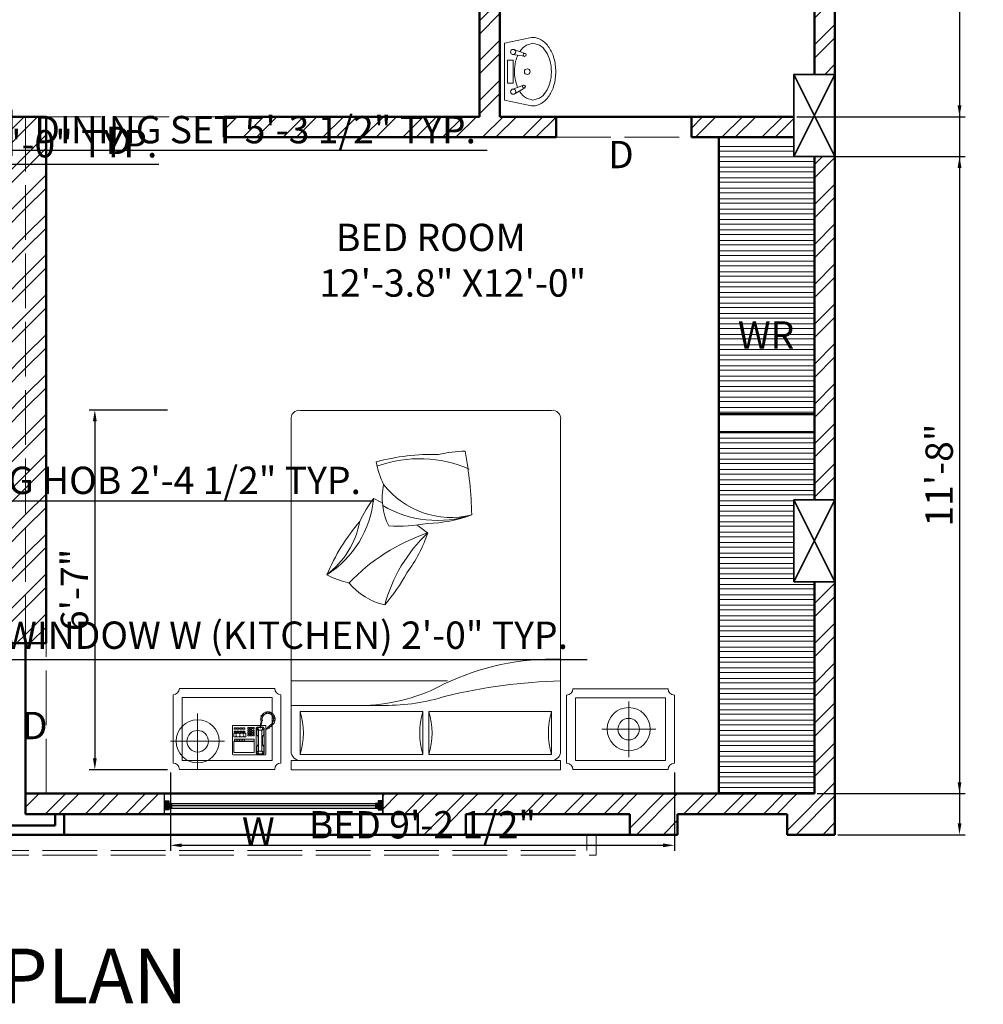
# Model space of a CAD drawing. Units: millimetres. Extents: x 4237 to 5109, y 21391 to 22486.
# Tile 14 of 17: x 4894 to 5105, y 21940 to 22156. Entities that reach past the tile are written whole.
import ezdxf

# ---------------------------------------------------------------- set-up
doc = ezdxf.new("R2010")
doc.units = ezdxf.units.MM
doc.linetypes.add('ACAD_ISO02W100', pattern=[15, 12, -3])
for name, color, linetype, lineweight in [('A-ANNO-DIMS', 2, 'Continuous', 18), ('A-ANNO-TEXT', 7, 'Continuous', 18), ('A-AREA-IDEN', 3, 'Continuous', 18), ('A-FLOR-OVHD', 1, 'ACAD_ISO02W100', 18), ('A-FURN', 8, 'Continuous', 18), ('A-FURN-CASE', 31, 'Continuous', 13), ('A-WALL', 7, 'Continuous', 50), ('A-WALL-PATT', 252, 'Continuous', 13), ('column', 102, 'Continuous', 35), ('windows', 140, 'Continuous', 25)]:
    doc.layers.add(name, color=color, linetype=linetype, lineweight=lineweight)
doc.styles.get("Standard").update_dxf_attribs({"font": 'arial.ttf'})
doc.dimstyles.new('ISO-25', dxfattribs={"dimtxt": 6, "dimasz": 2.5, "dimexe": 1.25, "dimexo": 0.625, "dimtad": 1, "dimdec": 1, "dimlunit": 4, "dimtxsty": 'Standard', "dimcen": 2.5, "dimadec": 0, "dimazin": 0, "dimtfac": 1, "dimtdec": 1, "dimtmove": 0, "dimatfit": 3, "dimfxl": 1, "dimarcsym": 0})

# ---------------------------------------------------------------- blocks, each defined once
blk = doc.blocks.new('A$C60F95712')
for p, q in [((0.05, 0.45), (0.003, 0.2283)), ((0.55, 0.45), (0.05, 0.45)), ((0.597, 0.2283), (0.55, 0.45)), ((0.1035, 0.3639), (0.1588, 0.2727)), ((0.1448, 0.3831), (0.1814, 0.2836)), ((0.4, 0.425), (0.2, 0.425)), ((0.2, 0.425), (0.2, 0.375)), ((0.2, 0.375), (0.4, 0.375)), ((0.4, 0.375), (0.4, 0.425)), ((0.4514, 0.3804), (0.4348, 0.2751)), ((0.4953, 0.3684), (0.459, 0.2688))]:
    blk.add_line(p, q)
for points in [[(0.4439, 0.3328, 0.046779), (0.3911, 0.3524, 0.080145), (0.3, 0.3617, 0.065516), (0.2003, 0.3485, 0.037125), (0.1623, 0.3353, 0.107176)], [(0.1307, 0.319, 0.008163), (0.1232, 0.3143, 0.107176), (0.0669, 0.2578), (0.05, 0.2), (0.0669, 0.1422, 0.107176), (0.1232, 0.0857, 0.078233), (0.2003, 0.0515, 0.065516), (0.3, 0.0383, 0.065516), (0.3997, 0.0515, 0.078233), (0.4768, 0.0857, 0.107176), (0.5331, 0.1422), (0.55, 0.2)], [(0.55, 0.2), (0.5331, 0.2578, 0.107176), (0.4768, 0.3143, 0.000976), (0.4758, 0.3149, 0.080145)]]:
    blk.add_lwpolyline(points, format="xyb")
for centre, radius in [((0.1241, 0.3735), 0.0228), ((0.4733, 0.3744), 0.0228), ((0.1696, 0.2793), 0.0126), ((0.3, 0.25), 0.025), ((0.4472, 0.2731), 0.0126)]:
    blk.add_circle(centre, radius)
for centre, radius, start, end in [((0.1362, 0.2), 0.1362, 168.02396, 180), ((0.1362, 0.2), 0.1362, 180, 211.85353), ((0.4638, 0.2), 0.1362, 328.14647, 0), ((0.4638, 0.2), 0.1362, 0, 11.97604), ((0.2147, 0.2488), 0.2286, 211.85353, 236.30993), ((0.3853, 0.2488), 0.2286, 303.69007, 328.14647), ((0.2662, 0.3261), 0.3215, 236.30993, 254.56292), ((0.3, 0.4484), 0.4484, 254.56292, 270), ((0.3, 0.4484), 0.4484, 270, 285.43708), ((0.3338, 0.3261), 0.3215, 285.43708, 303.69007)]:
    blk.add_arc(centre, radius, start, end)
blk = doc.blocks.new('A$C07097A50')
for p, q in [((0.0503, 1.9981), (0.5803, 1.9981)), ((0.1513, 1.6872), (0.1513, 1.9968)), ((0.6716, 1.9489), (0.6716, 2.0001)), ((0.6716, 2.0001), (2.1719, 2.0001)), ((2.1719, 1.9489), (2.1719, 2.0001)), ((2.7701, 1.9993), (2.2401, 1.9993)), ((0.0153, 1.9631), (0.0153, 1.5831)), ((0.0653, 1.9481), (0.0653, 1.5981)), ((0.0653, 1.9481), (0.5653, 1.9481)), ((0.5653, 1.9481), (0.5653, 1.5981)), ((0.6153, 1.9631), (0.6153, 1.5831)), ((2.1719, 1.9489), (0.6716, 1.9489)), ((2.2051, 1.9643), (2.2051, 1.5843)), ((2.2551, 1.9493), (2.2551, 1.5993)), ((2.7551, 1.9493), (2.2551, 1.9493)), ((2.5505, 1.6201), (2.5505, 1.9296)), ((2.7551, 1.9493), (2.7551, 1.5993)), ((2.8051, 1.9643), (2.8051, 1.5843)), ((0.3481, 1.9163), (0.3458, 1.914)), ((0.3458, 1.914), (0.3458, 1.7563)), ((0.3481, 1.9163), (0.5287, 1.9163)), ((0.3526, 1.9037), (0.3526, 1.8431)), ((0.4669, 1.9037), (0.3526, 1.9037)), ((0.4669, 1.8431), (0.4669, 1.9037)), ((0.4772, 1.9071), (0.4818, 1.9129)), ((0.4772, 1.7688), (0.4772, 1.9071)), ((0.4818, 1.9094), (0.4807, 1.9049)), ((0.4807, 1.9049), (0.4807, 1.874)), ((0.4807, 1.9049), (0.4909, 1.8946)), ((0.4807, 1.874), (0.4829, 1.8683)), ((0.4818, 1.9129), (0.5161, 1.9129)), ((0.4864, 1.9117), (0.4818, 1.9094)), ((0.4829, 1.8683), (0.4864, 1.8626)), ((0.4921, 1.8969), (0.4864, 1.9117)), ((0.4864, 1.9117), (0.5138, 1.9117)), ((0.4909, 1.8946), (0.4921, 1.8969)), ((0.4909, 1.8431), (0.4909, 1.8946)), ((0.5081, 1.8969), (0.4921, 1.8969)), ((0.5081, 1.8969), (0.5138, 1.9117)), ((0.5092, 1.8946), (0.5081, 1.8969)), ((0.5195, 1.9049), (0.5092, 1.8946)), ((0.5092, 1.8431), (0.5092, 1.8946)), ((0.5138, 1.9117), (0.5184, 1.9094)), ((0.5172, 1.8683), (0.5138, 1.8626)), ((0.5161, 1.9129), (0.5218, 1.9071)), ((0.5195, 1.874), (0.5172, 1.8683)), ((0.5184, 1.9094), (0.5195, 1.9049)), ((0.5195, 1.9049), (0.5195, 1.874)), ((0.5218, 1.9071), (0.5218, 1.77)), ((0.5287, 1.9163), (0.5309, 1.914)), ((0.5309, 1.914), (0.5309, 1.7563)), ((0.6716, 1.8977), (0.6716, 0.0512)), ((2.1719, 0.0512), (2.1719, 1.8977)), ((0, 1.8416), (0.3001, 1.8416)), ((0.3526, 1.8431), (0.4669, 1.8431)), ((0.4201, 1.8168), (0.3526, 1.8168)), ((0.3526, 1.8168), (0.3526, 1.7963)), ((0.3572, 1.8409), (0.3572, 1.8294)), ((0.4669, 1.8409), (0.3572, 1.8409)), ((0.3572, 1.8294), (0.4669, 1.8294)), ((0.3675, 1.8146), (0.3641, 1.8146)), ((0.3641, 1.8146), (0.3641, 1.8111)), ((0.3641, 1.8111), (0.3675, 1.8111)), ((0.3664, 1.8409), (0.3664, 1.8294)), ((0.3675, 1.8111), (0.3675, 1.8146)), ((0.3755, 1.8409), (0.3755, 1.8294)), ((0.3846, 1.8409), (0.3846, 1.8294)), ((0.3846, 1.8146), (0.3846, 1.8111)), ((0.3881, 1.8146), (0.3846, 1.8146)), ((0.3846, 1.8111), (0.3881, 1.8111)), ((0.3881, 1.8111), (0.3881, 1.8146)), ((0.3938, 1.8409), (0.3938, 1.8294)), ((0.4029, 1.8409), (0.4029, 1.8294)), ((0.4052, 1.8146), (0.4052, 1.8111)), ((0.4086, 1.8146), (0.4052, 1.8146)), ((0.4052, 1.8111), (0.4086, 1.8111)), ((0.4086, 1.8111), (0.4086, 1.8146)), ((0.4121, 1.8409), (0.4121, 1.8294)), ((0.4201, 1.7963), (0.4201, 1.8168)), ((0.4304, 1.8111), (0.4395, 1.8111)), ((0.4304, 1.8043), (0.4304, 1.8111)), ((0.4395, 1.8111), (0.4395, 1.8043)), ((0.4441, 1.8043), (0.4441, 1.8111)), ((0.4441, 1.8111), (0.4532, 1.8111)), ((0.4532, 1.8111), (0.4532, 1.8043)), ((0.4578, 1.8111), (0.4669, 1.8111)), ((0.4578, 1.8043), (0.4578, 1.8111)), ((0.4669, 1.8294), (0.4669, 1.8409)), ((0.4669, 1.8111), (0.4669, 1.8043)), ((0.4829, 1.8077), (0.4864, 1.8134)), ((0.4864, 1.8626), (0.4875, 1.8546)), ((0.4864, 1.8134), (0.4875, 1.8214)), ((0.4875, 1.8546), (0.4875, 1.8431)), ((0.4875, 1.8214), (0.4875, 1.8431)), ((0.4909, 1.8431), (0.4909, 1.7814)), ((0.5092, 1.8431), (0.5092, 1.7814)), ((0.5138, 1.8626), (0.5127, 1.8546)), ((0.5127, 1.8546), (0.5127, 1.8431)), ((0.5127, 1.8214), (0.5127, 1.8431)), ((0.5138, 1.8134), (0.5127, 1.8214)), ((0.5172, 1.8077), (0.5138, 1.8134)), ((0.3458, 1.7563), (0.3481, 1.754)), ((0.5, 1.754), (0.3481, 1.754)), ((0.3526, 1.7963), (0.4201, 1.7963)), ((0.3652, 1.7906), (0.3538, 1.7906)), ((0.3538, 1.7906), (0.3538, 1.786)), ((0.3538, 1.786), (0.3652, 1.786)), ((0.3538, 1.7666), (0.3538, 1.7734)), ((0.3538, 1.7734), (0.3652, 1.7734)), ((0.3652, 1.7666), (0.3538, 1.7666)), ((0.3641, 1.802), (0.3641, 1.7986)), ((0.3675, 1.802), (0.3641, 1.802)), ((0.3641, 1.7986), (0.3675, 1.7986)), ((0.3652, 1.786), (0.3652, 1.7906)), ((0.3652, 1.7734), (0.3652, 1.7666)), ((0.3675, 1.7986), (0.3675, 1.802)), ((0.3812, 1.7906), (0.3698, 1.7906)), ((0.3698, 1.7906), (0.3698, 1.786)), ((0.3698, 1.786), (0.3812, 1.786)), ((0.3698, 1.7666), (0.3698, 1.7734)), ((0.3698, 1.7734), (0.3812, 1.7734)), ((0.3812, 1.7666), (0.3698, 1.7666)), ((0.3812, 1.786), (0.3812, 1.7906)), ((0.3812, 1.7734), (0.3812, 1.7666)), ((0.3846, 1.802), (0.3846, 1.7986)), ((0.3881, 1.802), (0.3846, 1.802)), ((0.3846, 1.7986), (0.3881, 1.7986)), ((0.3972, 1.7906), (0.3858, 1.7906)), ((0.3858, 1.7906), (0.3858, 1.786)), ((0.3858, 1.786), (0.3972, 1.786)), ((0.3858, 1.7666), (0.3858, 1.7734)), ((0.3858, 1.7734), (0.3972, 1.7734)), ((0.3972, 1.7666), (0.3858, 1.7666)), ((0.3881, 1.7986), (0.3881, 1.802)), ((0.3972, 1.786), (0.3972, 1.7906)), ((0.3972, 1.7734), (0.3972, 1.7666)), ((0.4018, 1.7906), (0.4018, 1.786)), ((0.4132, 1.7906), (0.4018, 1.7906)), ((0.4018, 1.786), (0.4132, 1.786)), ((0.4018, 1.7734), (0.4132, 1.7734)), ((0.4018, 1.7666), (0.4018, 1.7734)), ((0.4132, 1.7666), (0.4018, 1.7666)), ((0.4052, 1.802), (0.4052, 1.7986)), ((0.4086, 1.802), (0.4052, 1.802)), ((0.4052, 1.7986), (0.4086, 1.7986)), ((0.4086, 1.7986), (0.4086, 1.802)), ((0.4132, 1.786), (0.4132, 1.7906)), ((0.4132, 1.7734), (0.4132, 1.7666)), ((0.4395, 1.8043), (0.4304, 1.8043)), ((0.4304, 1.7986), (0.4395, 1.7986)), ((0.4304, 1.7917), (0.4304, 1.7986)), ((0.4395, 1.7917), (0.4304, 1.7917)), ((0.4304, 1.778), (0.4304, 1.7848)), ((0.4304, 1.7848), (0.4395, 1.7848)), ((0.4395, 1.778), (0.4304, 1.778)), ((0.4304, 1.7723), (0.4395, 1.7723)), ((0.4304, 1.7654), (0.4304, 1.7723)), ((0.4395, 1.7654), (0.4304, 1.7654)), ((0.4395, 1.7986), (0.4395, 1.7917)), ((0.4395, 1.7848), (0.4395, 1.778)), ((0.4395, 1.7723), (0.4395, 1.7654)), ((0.4532, 1.8043), (0.4441, 1.8043)), ((0.4441, 1.7986), (0.4532, 1.7986)), ((0.4441, 1.7917), (0.4441, 1.7986)), ((0.4532, 1.7917), (0.4441, 1.7917)), ((0.4441, 1.778), (0.4441, 1.7848)), ((0.4441, 1.7848), (0.4532, 1.7848)), ((0.4532, 1.778), (0.4441, 1.778)), ((0.4441, 1.7723), (0.4532, 1.7723)), ((0.4441, 1.7654), (0.4441, 1.7723)), ((0.4532, 1.7654), (0.4441, 1.7654)), ((0.4532, 1.7986), (0.4532, 1.7917)), ((0.4532, 1.7848), (0.4532, 1.778)), ((0.4532, 1.7723), (0.4532, 1.7654)), ((0.4669, 1.8043), (0.4578, 1.8043)), ((0.4578, 1.7986), (0.4669, 1.7986)), ((0.4578, 1.7917), (0.4578, 1.7986)), ((0.4669, 1.7917), (0.4578, 1.7917)), ((0.4578, 1.7791), (0.4578, 1.786)), ((0.4578, 1.786), (0.4669, 1.786)), ((0.4669, 1.7791), (0.4578, 1.7791)), ((0.4578, 1.7654), (0.4578, 1.7723)), ((0.4578, 1.7723), (0.4669, 1.7723)), ((0.4669, 1.7654), (0.4578, 1.7654)), ((0.4669, 1.7986), (0.4669, 1.7917)), ((0.4669, 1.786), (0.4669, 1.7791)), ((0.4669, 1.7723), (0.4669, 1.7654)), ((0.4829, 1.7631), (0.4772, 1.7688)), ((0.4807, 1.802), (0.4829, 1.8077)), ((0.4807, 1.7711), (0.4807, 1.802)), ((0.4807, 1.7711), (0.4909, 1.7814)), ((0.4818, 1.7666), (0.4807, 1.7711)), ((0.4864, 1.7643), (0.4818, 1.7666)), ((0.499, 1.7631), (0.4829, 1.7631)), ((0.4921, 1.7791), (0.4864, 1.7643)), ((0.4864, 1.7643), (0.499, 1.7643)), ((0.4909, 1.7814), (0.4921, 1.7791)), ((0.5081, 1.7791), (0.4921, 1.7791)), ((0.5024, 1.7677), (0.4989, 1.7677)), ((0.4989, 1.7677), (0.4991, 1.7578)), ((0.4991, 1.7578), (0.5019, 1.7463)), ((0.503, 1.7585), (0.5024, 1.7677)), ((0.5026, 1.7643), (0.5138, 1.7643)), ((0.5161, 1.7631), (0.5027, 1.7631)), ((0.5047, 1.7511), (0.503, 1.7585)), ((0.5287, 1.754), (0.504, 1.754)), ((0.5092, 1.7814), (0.5081, 1.7791)), ((0.5081, 1.7791), (0.5138, 1.7643)), ((0.5195, 1.7711), (0.5092, 1.7814)), ((0.5138, 1.7643), (0.5184, 1.7666)), ((0.5218, 1.77), (0.5161, 1.7631)), ((0.5195, 1.802), (0.5172, 1.8077)), ((0.5184, 1.7666), (0.5195, 1.7711)), ((0.5195, 1.7711), (0.5195, 1.802)), ((0.5309, 1.7563), (0.5287, 1.754)), ((0.5378, 1.7743), (0.5309, 1.7768)), ((0.5309, 1.7723), (0.536, 1.7709)), ((0.536, 1.7709), (0.5406, 1.7672)), ((0.541, 1.7711), (0.5378, 1.7743)), ((0.5406, 1.7672), (0.5418, 1.7656)), ((0.5434, 1.7689), (0.541, 1.7711)), ((0.5442, 1.7658), (0.5418, 1.7634)), ((0.5418, 1.7656), (0.5442, 1.7658)), ((0.5418, 1.7634), (0.5511, 1.7552)), ((0.5477, 1.7705), (0.5434, 1.7689)), ((0.5497, 1.7685), (0.5477, 1.7705)), ((0.5481, 1.765), (0.5497, 1.7685)), ((0.5509, 1.7672), (0.5481, 1.765)), ((0.5539, 1.764), (0.5509, 1.7672)), ((0.5511, 1.7552), (0.5662, 1.7423)), ((0.5515, 1.7574), (0.5539, 1.764)), ((0.5577, 1.7606), (0.5515, 1.7574)), ((0.563, 1.7556), (0.5577, 1.7606)), ((0.5618, 1.7483), (0.563, 1.7556)), ((2.7018, 1.7745), (2.4017, 1.7745)), ((0.5019, 1.7463), (0.5047, 1.7354)), ((0.5026, 1.7254), (0.5021, 1.7199)), ((0.5021, 1.7199), (0.5088, 1.7187)), ((0.5088, 1.7187), (0.5023, 1.7148)), ((0.5023, 1.7148), (0.5028, 1.7085)), ((0.5051, 1.728), (0.5026, 1.7254)), ((0.5028, 1.7085), (0.5102, 1.7078)), ((0.5102, 1.7078), (0.5037, 1.7028)), ((0.5037, 1.7028), (0.5067, 1.6974)), ((0.5047, 1.7354), (0.5044, 1.7294)), ((0.5044, 1.7294), (0.5051, 1.728)), ((0.5074, 1.7403), (0.5047, 1.7511)), ((0.5067, 1.6974), (0.5137, 1.6988)), ((0.5081, 1.7347), (0.5074, 1.7403)), ((0.5079, 1.7287), (0.5081, 1.7347)), ((0.5121, 1.7257), (0.5079, 1.7287)), ((0.5137, 1.6988), (0.5104, 1.6923)), ((0.5111, 1.7203), (0.5121, 1.7257)), ((0.5123, 1.7058), (0.5111, 1.7203)), ((0.5211, 1.6947), (0.5123, 1.7058)), ((0.5708, 1.7028), (0.5606, 1.6928)), ((0.567, 1.7515), (0.5618, 1.7483)), ((0.5664, 1.7419), (0.574, 1.7201)), ((0.5714, 1.7469), (0.567, 1.7515)), ((0.5696, 1.7419), (0.5714, 1.7469)), ((0.5766, 1.7426), (0.5697, 1.7419)), ((0.574, 1.7201), (0.5708, 1.7028)), ((0.5745, 1.6926), (0.5713, 1.6988)), ((0.5713, 1.6988), (0.578, 1.6967)), ((0.572, 1.7331), (0.5787, 1.7356)), ((0.5794, 1.7333), (0.572, 1.7331)), ((0.5743, 1.7076), (0.5814, 1.7074)), ((0.5798, 1.7014), (0.5743, 1.7076)), ((0.5761, 1.7234), (0.581, 1.728)), ((0.5824, 1.7234), (0.5761, 1.7234)), ((0.5764, 1.7155), (0.5835, 1.7176)), ((0.5824, 1.712), (0.5764, 1.7155)), ((0.5787, 1.7356), (0.5766, 1.7426)), ((0.578, 1.6967), (0.5798, 1.7014)), ((0.581, 1.728), (0.5794, 1.7333)), ((0.5814, 1.7074), (0.5824, 1.712)), ((0.5835, 1.7176), (0.5824, 1.7234)), ((0.5104, 1.6923), (0.5139, 1.6882)), ((0.5139, 1.6882), (0.5192, 1.6921)), ((0.5192, 1.6921), (0.5183, 1.6859)), ((0.5183, 1.6859), (0.5227, 1.6831)), ((0.5333, 1.6882), (0.5211, 1.6947)), ((0.5227, 1.6831), (0.5282, 1.6877)), ((0.5282, 1.6877), (0.5276, 1.6801)), ((0.5276, 1.6801), (0.5324, 1.6787)), ((0.5324, 1.6787), (0.5354, 1.6849)), ((0.5472, 1.687), (0.5333, 1.6882)), ((0.5354, 1.6849), (0.5382, 1.6787)), ((0.5382, 1.6787), (0.5421, 1.6782)), ((0.5421, 1.6782), (0.5437, 1.6849)), ((0.5437, 1.6849), (0.5463, 1.6775)), ((0.5463, 1.6775), (0.5507, 1.6787)), ((0.5606, 1.6928), (0.5472, 1.687)), ((0.5507, 1.6787), (0.5509, 1.6849)), ((0.5509, 1.6849), (0.5562, 1.6803)), ((0.5562, 1.6803), (0.5599, 1.6822)), ((0.5592, 1.6891), (0.5641, 1.6831)), ((0.5599, 1.6822), (0.5592, 1.6891)), ((0.5641, 1.6831), (0.5678, 1.6863)), ((0.565, 1.6926), (0.5715, 1.6898)), ((0.5678, 1.6863), (0.565, 1.6926)), ((0.5715, 1.6898), (0.5745, 1.6926)), ((0.0653, 1.5981), (0.5653, 1.5981)), ((2.7551, 1.5993), (2.2551, 1.5993)), ((0.0503, 1.5481), (0.5803, 1.5481)), ((2.7701, 1.5493), (2.2401, 1.5493)), ((0.7228, 0.0001), (2.1207, 0.0001))]:
    blk.add_line(p, q)
at = {"linetype": 'ByBlock'}
for p, q in [((0.7228, 1.6759), (0.7228, 1.9148)), ((0.7228, 1.9148), (1.4047, 1.9148)), ((1.4047, 1.9148), (1.4047, 1.6759)), ((1.4388, 1.6759), (1.4388, 1.9148)), ((1.4388, 1.9148), (2.1207, 1.9148)), ((2.1207, 1.9148), (2.1207, 1.6759)), ((1.4047, 1.6759), (0.7228, 1.6759)), ((2.1207, 1.6759), (1.4388, 1.6759)), ((1.1914, 1.6418), (0.6716, 1.6418)), ((1.5412, 1.5053), (0.6716, 1.5053))]:
    blk.add_line(p, q, dxfattribs=at)
for centre in [(0.1513, 1.8416), (2.5505, 1.7745)]:
    blk.add_circle(centre, 0.12, dxfattribs=at)
for centre in [(0.1513, 1.8416), (2.5505, 1.7745)]:
    blk.add_circle(centre, 0.06)
for centre, radius, start, end in [((0.0153, 1.9981), 0.035, 270, 0), ((0.6153, 1.9981), 0.035, 180, 270), ((2.2051, 1.9993), 0.035, 270, 0), ((2.8051, 1.9993), 0.035, 180, 270), ((0.7228, 1.8977), 0.0512, 90, 180), ((2.1207, 1.8977), 0.0512, 0, 90), ((0.0153, 1.5481), 0.035, 0, 90), ((0.6153, 1.5481), 0.035, 90, 180), ((2.2051, 1.5493), 0.035, 0, 90), ((2.8051, 1.5493), 0.035, 90, 180), ((1.2698, 0.7333), 0.3575, 102.4782, 140.4625), ((0.4476, 0.4335), 0.9879, 28.4971, 41.0566), ((2.0313, 1.3124), 0.8697, 195.336, 226.4193), ((1.1192, 0.4274), 0.548, 103.2034, 117.0362), ((1.7756, 1.7059), 1.0798, 223.6306, 251.4288), ((1.9422, 1.372), 1.1652, 203.0642, 220.3209), ((0.5744, 0.5274), 0.4879, 10.6986, 52.6864), ((0.5678, 0.4375), 0.5655, 5.3391, 57.6895), ((0.6844, 0.4345), 0.7874, 18.3527, 36.6851), ((0.1017, 2.4319), 2.1977, 305.2966, 307.2418), ((1.7177, 0.9312), 0.734, 205.259, 216.9351), ((1.5362, 0.487), 0.3575, 154.0418, 192.0262), ((1.4868, 0.0041), 0.6085, 71.81, 120.1351), ((1.2599, -0.3434), 0.9879, 80.0607, 92.6202), ((1.4063, -0.1573), 0.7874, 69.9163, 88.2487), ((1.5627, 0.1186), 0.4774, 76.1849, 142.0017), ((-0.5205, 0.628), 2.1977, 349.4884, 358.8054), ((0.1017, 2.4319), 2.1977, 297.9248, 299.3793), ((1.6822, 0.1789), 0.548, 154.767, 168.5998), ((1.4539, 1.4107), 1.1652, 254.6278, 271.8845), ((1.3874, 0.9578), 0.6885, 250.2936, 293.6414), ((1.6595, 0.9609), 0.734, 256.8226, 268.4988), ((0.717, 0.0455), 0.0458, 172.7599, 277.2401), ((2.1265, 0.0455), 0.0458, 262.7599, 7.2401)]:
    blk.add_arc(centre, radius, start, end)
for centre, radius, start, end in [((0.3133, 1.7953), 0.4265, 343.7398, 16.2602), ((1.8141, 1.7953), 0.4265, 163.7398, 196.2602), ((1.0294, 1.7953), 0.4265, 343.7398, 16.2602), ((2.5302, 1.7953), 0.4265, 163.7398, 196.2602), ((1.053, 0.6571), 0.9853, 61.4328, 88.1261), ((1.2053, 0.5713), 1.0706, 72.1966, 90.7418), ((2.2595, 4.5996), 3.0955, 256.4201, 268.3789), ((2.1283, 2.7745), 1.3903, 244.2427, 271.7984)]:
    blk.add_arc(centre, radius, start, end, dxfattribs=at)
blk = doc.blocks.new('COLUMN-X')
blk.add_line((18, 9), (0, 0))
blk.add_lwpolyline([(18, 9), (0, 9), (0, 0), (18, 0)], close=True)
blk = doc.blocks.new('*D72')
at = {"layer": 'A-ANNO-DIMS', "color": 0, "lineweight": -2, "transparency": 16777216}
for p, q in [((4926.7, 21990.83), (4926.7, 21973.62)), ((5037.29, 21990.83), (5037.29, 21973.62)), ((4929.2, 21974.87), (5034.79, 21974.87))]:
    blk.add_line(p, q, dxfattribs=at)
at = {"layer": 'A-ANNO-DIMS', "color": 0, "transparency": 16777216}
for points in [[(4929.2, 21975.28), (4929.2, 21974.45), (4926.7, 21974.87)], [(5034.79, 21975.28), (5034.79, 21974.45), (5037.29, 21974.87)]]:
    blk.add_solid(points, dxfattribs=at)
at = {"layer": 'Defpoints', "color": 0, "transparency": 16777216}
for p in [(4926.7, 21991.46), (5037.29, 21991.46), (5037.29, 21974.87)]:
    blk.add_point(p, dxfattribs=at)
at = {"layer": 'A-ANNO-DIMS', "color": 0, "transparency": 16777216, "insert": (4982, 21978.59), "char_height": 6, "attachment_point": 5}
blk.add_mtext('BED 9\'-2 1/2"', dxfattribs=at)
blk = doc.blocks.new('*D73')
at = {"layer": 'A-ANNO-DIMS', "color": 0, "lineweight": -2, "transparency": 16777216}
for p, q in [((4926.08, 22070.37), (4908.87, 22070.37)), ((4910.12, 22067.87), (4910.12, 21993.96)), ((4926.08, 21991.46), (4908.87, 21991.46))]:
    blk.add_line(p, q, dxfattribs=at)
at = {"layer": 'A-ANNO-DIMS', "color": 0, "transparency": 16777216}
for points in [[(4909.7, 22067.87), (4910.53, 22067.87), (4910.12, 22070.37)], [(4909.7, 21993.96), (4910.53, 21993.96), (4910.12, 21991.46)]]:
    blk.add_solid(points, dxfattribs=at)
at = {"layer": 'Defpoints', "color": 0, "transparency": 16777216}
for p in [(4926.7, 22070.37), (4910.12, 21991.46), (4926.7, 21991.46)]:
    blk.add_point(p, dxfattribs=at)
at = {"layer": 'A-ANNO-DIMS', "color": 0, "transparency": 16777216, "insert": (4906.43, 22030.91), "char_height": 6, "attachment_point": 5, "rotation": 90}
blk.add_mtext('6\'-7"', dxfattribs=at)
blk = doc.blocks.new('*D82')
at = {"layer": 'A-ANNO-DIMS', "color": 0, "lineweight": -2, "transparency": 16777216}
for p, q in [((4859.72, 22018.58), (4859.72, 22014.38)), ((4883.52, 22018.58), (4883.52, 22014.38)), ((4862.22, 22015.63), (4881.02, 22015.63)), ((4883.52, 22015.63), (5018.13, 22015.63))]:
    blk.add_line(p, q, dxfattribs=at)
at = {"layer": 'A-ANNO-DIMS', "color": 0, "transparency": 16777216}
for points in [[(4862.22, 22016.05), (4862.22, 22015.21), (4859.72, 22015.63)], [(4881.02, 22016.05), (4881.02, 22015.21), (4883.52, 22015.63)]]:
    blk.add_solid(points, dxfattribs=at)
at = {"layer": 'Defpoints', "color": 0, "transparency": 16777216}
for p in [(4859.72, 22019.2), (4883.52, 22019.2), (4883.52, 22015.63)]:
    blk.add_point(p, dxfattribs=at)
at = {"layer": 'A-ANNO-DIMS', "color": 0, "transparency": 16777216, "insert": (4952.07, 22020.19), "char_height": 6, "attachment_point": 5}
blk.add_mtext('WINDOW W (KITCHEN) 2\'-0" TYP.', dxfattribs=at)
blk = doc.blocks.new('*D86')
at = {"layer": 'A-ANNO-DIMS', "color": 0, "lineweight": -2, "transparency": 16777216}
for p, q in [((4826.09, 22046.76), (4826.09, 22051.68)), ((4828.59, 22050.43), (4852.22, 22050.43)), ((4854.72, 22046.76), (4854.72, 22051.68)), ((4854.72, 22050.43), (4971.36, 22050.43))]:
    blk.add_line(p, q, dxfattribs=at)
at = {"layer": 'A-ANNO-DIMS', "color": 0, "transparency": 16777216}
for points in [[(4828.59, 22050.85), (4828.59, 22050.02), (4826.09, 22050.43)], [(4852.22, 22050.85), (4852.22, 22050.02), (4854.72, 22050.43)]]:
    blk.add_solid(points, dxfattribs=at)
at = {"layer": 'Defpoints', "color": 0, "transparency": 16777216}
for p in [(4854.72, 22050.43), (4826.09, 22046.14), (4854.72, 22046.14)]:
    blk.add_point(p, dxfattribs=at)
at = {"layer": 'A-ANNO-DIMS', "color": 0, "transparency": 16777216, "insert": (4914.29, 22054.16), "char_height": 6, "attachment_point": 5}
blk.add_mtext('COOKING HOB 2\'-4 1/2" TYP.', dxfattribs=at)
blk = doc.blocks.new('*D89')
at = {"layer": 'A-ANNO-DIMS', "color": 0, "lineweight": -2, "transparency": 16777216}
for p, q in [((4872.25, 22121.32), (4872.25, 22125.58)), ((4884.39, 22121.32), (4884.39, 22125.58)), ((4874.75, 22124.33), (4881.89, 22124.33)), ((4884.39, 22124.33), (4924.15, 22124.33))]:
    blk.add_line(p, q, dxfattribs=at)
at = {"layer": 'A-ANNO-DIMS', "color": 0, "transparency": 16777216}
for points in [[(4874.75, 22124.75), (4874.75, 22123.92), (4872.25, 22124.33)], [(4881.89, 22124.75), (4881.89, 22123.92), (4884.39, 22124.33)]]:
    blk.add_solid(points, dxfattribs=at)
at = {"layer": 'Defpoints', "color": 0, "transparency": 16777216}
for p in [(4884.39, 22124.33), (4872.25, 22120.69), (4884.39, 22120.69)]:
    blk.add_point(p, dxfattribs=at)
at = {"layer": 'A-ANNO-DIMS', "color": 0, "transparency": 16777216, "insert": (4905.52, 22128.02), "char_height": 6, "attachment_point": 5}
blk.add_mtext('1\'-0" TYP.', dxfattribs=at)
blk = doc.blocks.new('*D92')
at = {"layer": 'A-ANNO-DIMS', "color": 0, "lineweight": -2, "transparency": 16777216}
for p, q in [((4828.57, 22136.25), (4828.57, 22126.13)), ((4891.89, 22136.25), (4891.89, 22126.13)), ((4831.07, 22127.38), (4889.39, 22127.38)), ((4891.89, 22127.38), (4996.19, 22127.38))]:
    blk.add_line(p, q, dxfattribs=at)
at = {"layer": 'A-ANNO-DIMS', "color": 0, "transparency": 16777216}
for points in [[(4831.07, 22127.8), (4831.07, 22126.96), (4828.57, 22127.38)], [(4889.39, 22127.8), (4889.39, 22126.96), (4891.89, 22127.38)]]:
    blk.add_solid(points, dxfattribs=at)
at = {"layer": 'Defpoints', "color": 0, "transparency": 16777216}
for p in [(4828.57, 22136.88), (4891.89, 22136.88), (4891.89, 22127.38)]:
    blk.add_point(p, dxfattribs=at)
at = {"layer": 'A-ANNO-DIMS', "color": 0, "transparency": 16777216, "insert": (4945.29, 22131.11), "char_height": 6, "attachment_point": 5}
blk.add_mtext('DINING SET 5\'-3 1/2" TYP.', dxfattribs=at)
blk = doc.blocks.new('*D116')
at = {"layer": 'A-ANNO-DIMS', "color": 0, "lineweight": -2, "transparency": 16777216}
for p, q in [((5073.14, 22440.7), (5101.11, 22440.7)), ((5099.86, 22438.2), (5099.86, 21979.7)), ((5073.14, 21977.2), (5101.11, 21977.2))]:
    blk.add_line(p, q, dxfattribs=at)
at = {"layer": 'A-ANNO-DIMS', "color": 0, "transparency": 16777216}
for points in [[(5099.45, 22438.2), (5100.28, 22438.2), (5099.86, 22440.7)], [(5099.45, 21979.7), (5100.28, 21979.7), (5099.86, 21977.2)]]:
    blk.add_solid(points, dxfattribs=at)
at = {"layer": 'Defpoints', "color": 0, "transparency": 16777216}
for p in [(5072.51, 22440.7), (5072.51, 21977.2), (5099.86, 21977.2)]:
    blk.add_point(p, dxfattribs=at)
at = {"layer": 'A-ANNO-DIMS', "color": 0, "transparency": 16777216, "insert": (5096.13, 22208.95), "char_height": 6, "attachment_point": 5, "rotation": 90}
blk.add_mtext('38\'-7 1/2"', dxfattribs=at)
blk = doc.blocks.new('*D118')
at = {"layer": 'A-ANNO-DIMS', "color": 0, "lineweight": -2, "transparency": 16777216}
for p, q in [((5068.64, 22283.2), (5101.11, 22283.2)), ((5099.86, 22280.7), (5099.86, 22137.2)), ((5064.14, 22134.7), (5101.11, 22134.7))]:
    blk.add_line(p, q, dxfattribs=at)
at = {"layer": 'A-ANNO-DIMS', "color": 0, "transparency": 16777216}
for points in [[(5099.45, 22280.7), (5100.28, 22280.7), (5099.86, 22283.2)], [(5099.45, 22137.2), (5100.28, 22137.2), (5099.86, 22134.7)]]:
    blk.add_solid(points, dxfattribs=at)
at = {"layer": 'Defpoints', "color": 0, "transparency": 16777216}
for p in [(5068.01, 22283.2), (5063.51, 22134.7), (5099.86, 22134.7)]:
    blk.add_point(p, dxfattribs=at)
at = {"layer": 'A-ANNO-DIMS', "color": 0, "transparency": 16777216, "insert": (5096.13, 22208.95), "char_height": 6, "attachment_point": 5, "rotation": 90}
blk.add_mtext('12\'-4 1/2"', dxfattribs=at)
blk = doc.blocks.new('*D119')
at = {"layer": 'A-ANNO-DIMS', "color": 0, "lineweight": -2, "transparency": 16777216}
for p, q in [((5068.64, 22126), (5101.11, 22126)), ((5099.86, 22123.5), (5099.86, 21988.7)), ((5068.64, 21986.2), (5101.11, 21986.2))]:
    blk.add_line(p, q, dxfattribs=at)
at = {"layer": 'A-ANNO-DIMS', "color": 0, "transparency": 16777216}
for points in [[(5099.45, 22123.5), (5100.28, 22123.5), (5099.86, 22126)], [(5099.45, 21988.7), (5100.28, 21988.7), (5099.86, 21986.2)]]:
    blk.add_solid(points, dxfattribs=at)
at = {"layer": 'Defpoints', "color": 0, "transparency": 16777216}
for p in [(5068.01, 22126), (5068.01, 21986.2), (5099.86, 21986.2)]:
    blk.add_point(p, dxfattribs=at)
at = {"layer": 'A-ANNO-DIMS', "color": 0, "transparency": 16777216, "insert": (5096.17, 22056.1), "char_height": 6, "attachment_point": 5, "rotation": 90}
blk.add_mtext('11\'-8"', dxfattribs=at)

msp = doc.modelspace()

# ---------------------------------------------------------------- hatches: boundary and pattern name
at = {"layer": 'A-WALL-PATT'}
h = msp.add_hatch(dxfattribs=at)
h.set_pattern_fill('ANSI32', color=256, scale=0.65)
h.paths.add_polyline_path([(5045.51, 22223.2), (5051.51, 22223.2), (5051.51, 22227.7), (5041.01, 22227.7), (5041.01, 22211.2), (4999.01, 22211.2), (4999.01, 22283.2), (5017.01, 22283.2), (5017.01, 22287.7), (4965.41, 22287.7), (4965.41, 22283.2), (4994.51, 22283.2), (4994.51, 22134.7), (4938.41, 22134.7), (4938.41, 22130.2), (5011.33, 22130.2), (5011.33, 22134.7), (4999.01, 22134.7), (4999.01, 22206.7), (5041.01, 22206.7), (5041.01, 22190.2), (5051.51, 22190.2), (5051.51, 22194.7), (5045.51, 22194.7)])
h = msp.add_hatch(dxfattribs=at)
h.set_pattern_fill('ANSI32', color=256, scale=0.65)
h.paths.add_polyline_path([(5072.51, 22283.2), (5068.01, 22283.2), (5068.01, 22144), (5072.51, 22144)])
h = msp.add_hatch(dxfattribs=at)
h.set_pattern_fill('ANSI32', color=256, scale=0.65)
h.paths.add_polyline_path([(4894.91, 22134.7), (4820.61, 22134.7), (4820.61, 22130.2), (4890.41, 22130.2), (4890.41, 22028.2), (4883.52, 22028.2), (4883.52, 22019.2), (4894.91, 22019.2)])
h = msp.add_hatch(dxfattribs=at)
h.set_pattern_fill('ANSI32', color=256, scale=0.65)
h.paths.add_polyline_path([(4899.41, 22134.7), (4894.91, 22134.7), (4894.91, 22019.2), (4899.41, 22019.2)])
h = msp.add_hatch(dxfattribs=at)
h.set_pattern_fill('ANSI32', color=256, scale=0.65)
h.paths.add_polyline_path([(5063.51, 22134.7), (5041.02, 22134.7), (5041.02, 22130.2), (5063.51, 22130.2)], flags=17)
h = msp.add_hatch(dxfattribs=at)
h.set_pattern_fill('ANSI32', color=256, scale=0.65)
h.paths.add_polyline_path([(5072.51, 22126), (5068.01, 22126), (5068.01, 22050.7), (5072.51, 22050.7)])
h = msp.add_hatch(dxfattribs=at)
h.set_pattern_fill('ANSI32', color=256, scale=0.65)
h.paths.add_polyline_path([(5072.51, 22032.7), (5068.01, 22032.7), (5068.01, 21986.2), (4973.32, 21986.2), (4973.32, 21981.7), (4981.01, 21981.7), (4981.01, 21977.2), (4991.51, 21977.2), (4991.51, 21981.7), (5027.51, 21981.7), (5027.51, 21977.2), (5038.01, 21977.2), (5038.01, 21981.7), (5062.01, 21981.7), (5062.01, 21977.2), (5072.51, 21977.2)])
h = msp.add_hatch(dxfattribs=at)
h.set_pattern_fill('ANSI32', color=256, scale=0.65)
h.paths.add_polyline_path([(4925.32, 21986.2), (4894.91, 21986.2), (4894.91, 21981.7), (4925.32, 21981.7)])
h = msp.add_hatch(color=256, dxfattribs=at)
h.dxf.hatch_style = 1
h.paths.add_polyline_path([(4926.95, 21984.03), (4926.32, 21984.03), (4926.32, 21984.62), (4925.32, 21984.62), (4925.32, 21982.62), (4926.32, 21982.62), (4926.32, 21983.03), (4926.95, 21983.03)], flags=17)
h = msp.add_hatch(color=256, dxfattribs=at)
h.dxf.hatch_style = 1
h.paths.add_polyline_path([(4973.32, 21984.62), (4972.32, 21984.62), (4972.32, 21984.03), (4971.7, 21984.03), (4971.7, 21983.03), (4972.32, 21983.03), (4972.32, 21982.62), (4973.32, 21982.62)])

# ---------------------------------------------------------------- linework, layer by layer
at = {"layer": 'A-FLOR-OVHD'}
for p, q in [((4894.91, 22134.7), (4894.91, 22019.2)), ((4899.41, 22134.7), (4938.41, 22134.7)), ((5011.33, 22130.2), (5041.02, 22130.2)), ((4899.41, 21986.2), (4899.41, 22019.2)), ((5018.1, 21977.2), (5018.1, 21973.7)), ((5020.1, 21977.2), (5020.1, 21972.7)), ((4763.61, 21973.7), (5018.1, 21973.7)), ((4763.61, 21972.7), (5020.1, 21972.7))]:
    msp.add_line(p, q, dxfattribs=at)
at = {"layer": 'A-FURN-CASE'}
for p, q in [((5047.01, 22128.2), (5063.51, 22128.2)), ((5047.01, 22127.2), (5063.51, 22127.2)), ((5047.01, 22125.91), (5068.01, 22125.91)), ((5047.01, 22124.91), (5068.01, 22124.91)), ((5047.01, 22123.62), (5068.01, 22123.62)), ((5047.01, 22122.62), (5068.01, 22122.62)), ((5047.01, 22121.33), (5068.01, 22121.33)), ((5047.01, 22120.33), (5068.01, 22120.33)), ((5047.01, 22119.04), (5068.01, 22119.04)), ((5047.01, 22118.04), (5068.01, 22118.04)), ((5047.01, 22116.74), (5068.01, 22116.74)), ((5047.01, 22115.74), (5068.01, 22115.74)), ((5047.01, 22114.45), (5068.01, 22114.45)), ((5047.01, 22113.45), (5068.01, 22113.45)), ((5047.01, 22112.16), (5068.01, 22112.16)), ((5047.01, 22111.16), (5068.01, 22111.16)), ((5047.01, 22109.87), (5068.01, 22109.87)), ((5047.01, 22108.87), (5068.01, 22108.87)), ((5047.01, 22107.58), (5068.01, 22107.58)), ((5047.01, 22106.58), (5068.01, 22106.58)), ((5047.01, 22105.29), (5068.01, 22105.29)), ((5047.01, 22104.29), (5068.01, 22104.29)), ((5047.01, 22103), (5068.01, 22103)), ((5047.01, 22102), (5068.01, 22102)), ((5047.01, 22100.71), (5068.01, 22100.71)), ((5047.01, 22099.71), (5068.01, 22099.71)), ((5047.01, 22098.41), (5068.01, 22098.41)), ((5047.01, 22097.41), (5068.01, 22097.41)), ((5047.01, 22096.12), (5068.01, 22096.12)), ((5047.01, 22095.12), (5068.01, 22095.12)), ((5047.01, 22093.83), (5068.01, 22093.83)), ((5047.01, 22092.83), (5068.01, 22092.83)), ((5047.01, 22091.54), (5068.01, 22091.54)), ((5047.01, 22090.54), (5068.01, 22090.54)), ((5047.01, 22089.25), (5068.01, 22089.25)), ((5047.01, 22088.25), (5068.01, 22088.25)), ((5047.01, 22086.96), (5068.01, 22086.96)), ((5047.01, 22085.96), (5068.01, 22085.96)), ((5047.01, 22084.67), (5068.01, 22084.67)), ((5047.01, 22083.67), (5068.01, 22083.67)), ((5047.01, 22082.38), (5068.01, 22082.38)), ((5047.01, 22081.38), (5068.01, 22081.38)), ((5047.01, 22080.08), (5068.01, 22080.08)), ((5047.01, 22079.08), (5068.01, 22079.08)), ((5047.01, 22077.79), (5068.01, 22077.79)), ((5047.01, 22076.79), (5068.01, 22076.79)), ((5047.01, 22075.5), (5068.01, 22075.5)), ((5047.01, 22074.5), (5068.01, 22074.5)), ((5047.01, 22073.21), (5068.01, 22073.21)), ((5047.01, 22072.21), (5068.01, 22072.21)), ((5047.01, 22070.92), (5068.01, 22070.92)), ((5047.01, 22069.92), (5068.01, 22069.92)), ((5047.01, 22064.19), (5068.01, 22064.19)), ((5047.01, 22063.19), (5068.01, 22063.19)), ((5047.01, 22061.9), (5068.01, 22061.9)), ((5047.01, 22060.9), (5068.01, 22060.9)), ((5047.01, 22059.61), (5068.01, 22059.61)), ((5047.01, 22058.61), (5068.01, 22058.61)), ((5047.01, 22057.32), (5068.01, 22057.32)), ((5047.01, 22056.32), (5068.01, 22056.32)), ((5047.01, 22055.03), (5068.01, 22055.03)), ((5047.01, 22054.03), (5068.01, 22054.03)), ((5047.01, 22052.74), (5068.01, 22052.74)), ((5047.01, 22051.74), (5068.01, 22051.74)), ((5047.01, 22050.45), (5063.51, 22050.45)), ((5047.01, 22049.45), (5063.51, 22049.45)), ((5047.01, 22048.15), (5063.51, 22048.15)), ((5047.01, 22047.15), (5063.51, 22047.15)), ((5047.01, 22045.86), (5063.51, 22045.86)), ((5047.01, 22044.86), (5063.51, 22044.86)), ((5047.01, 22043.57), (5063.51, 22043.57)), ((5047.01, 22042.57), (5063.51, 22042.57)), ((5047.01, 22041.28), (5063.51, 22041.28)), ((5047.01, 22040.28), (5063.51, 22040.28)), ((5047.01, 22038.99), (5063.51, 22038.99)), ((5047.01, 22037.99), (5063.51, 22037.99)), ((5047.01, 22036.7), (5063.51, 22036.7)), ((5047.01, 22035.7), (5063.51, 22035.7)), ((5047.01, 22034.41), (5063.51, 22034.41)), ((5047.01, 22033.41), (5063.51, 22033.41)), ((5047.01, 22032.12), (5068.01, 22032.12)), ((5047.01, 22031.12), (5068.01, 22031.12)), ((5047.01, 22029.82), (5068.01, 22029.82)), ((5047.01, 22028.82), (5068.01, 22028.82)), ((5047.01, 22027.53), (5068.01, 22027.53)), ((5047.01, 22026.53), (5068.01, 22026.53)), ((5047.01, 22025.24), (5068.01, 22025.24)), ((5047.01, 22024.24), (5068.01, 22024.24)), ((5047.01, 22022.95), (5068.01, 22022.95)), ((5047.01, 22021.95), (5068.01, 22021.95)), ((5047.01, 22020.66), (5068.01, 22020.66)), ((5047.01, 22019.66), (5068.01, 22019.66)), ((5047.01, 22018.37), (5068.01, 22018.37)), ((5047.01, 22017.37), (5068.01, 22017.37)), ((5047.01, 22016.08), (5068.01, 22016.08)), ((5047.01, 22015.08), (5068.01, 22015.08)), ((5047.01, 22013.79), (5068.01, 22013.79)), ((5047.01, 22012.79), (5068.01, 22012.79)), ((5047.01, 22011.49), (5068.01, 22011.49)), ((5047.01, 22010.49), (5068.01, 22010.49)), ((5047.01, 22009.2), (5068.01, 22009.2)), ((5047.01, 22008.2), (5068.01, 22008.2)), ((5047.01, 22006.91), (5068.01, 22006.91)), ((5047.01, 22005.91), (5068.01, 22005.91)), ((5047.01, 22004.62), (5068.01, 22004.62)), ((5047.01, 22003.62), (5068.01, 22003.62)), ((5047.01, 22002.33), (5068.01, 22002.33)), ((5047.01, 22001.33), (5068.01, 22001.33)), ((5047.01, 22000.04), (5068.01, 22000.04)), ((5047.01, 21999.04), (5068.01, 21999.04)), ((5047.01, 21997.75), (5068.01, 21997.75)), ((5047.01, 21996.75), (5068.01, 21996.75)), ((5047.01, 21995.46), (5068.01, 21995.46)), ((5047.01, 21994.46), (5068.01, 21994.46)), ((5047.01, 21993.16), (5068.01, 21993.16)), ((5047.01, 21992.16), (5068.01, 21992.16)), ((5047.01, 21990.87), (5068.01, 21990.87)), ((5047.01, 21989.87), (5068.01, 21989.87)), ((5047.01, 21988.58), (5068.01, 21988.58)), ((5047.01, 21987.58), (5068.01, 21987.58))]:
    msp.add_line(p, q, dxfattribs=at)
at = {"layer": 'A-WALL'}
for p, q in [((5072.51, 22436.2), (5072.51, 21977.2)), ((4994.51, 22283.2), (4994.51, 22134.7)), ((5068.01, 22283.2), (5068.01, 22144)), ((4999.01, 22206.7), (4999.01, 22134.7)), ((4820.61, 22134.7), (4899.41, 22134.7)), ((4899.41, 22134.7), (4899.41, 22019.2)), ((4938.41, 22134.7), (4938.41, 22130.2)), ((4938.41, 22134.7), (4994.51, 22134.7)), ((4999.01, 22134.7), (5011.33, 22134.7)), ((5011.33, 22134.7), (5011.33, 22130.2)), ((5011.33, 22134.7), (5041.02, 22134.7)), ((5041.02, 22134.7), (5063.51, 22134.7)), ((5041.02, 22134.7), (5041.02, 22130.2)), ((4938.41, 22130.2), (5011.33, 22130.2)), ((5041.02, 22130.2), (5063.51, 22130.2)), ((5047.01, 22130.2), (5047.01, 21986.2)), ((5068.01, 22126), (5068.01, 22050.7)), ((5068.01, 22069.48), (5047.01, 22069.48)), ((5068.01, 22065.48), (5047.01, 22065.48)), ((5068.01, 22032.7), (5068.01, 21986.2)), ((4786.11, 22019.2), (4899.41, 22019.2)), ((4894.91, 22019.2), (4894.91, 21981.7)), ((4894.91, 21986.2), (5068.01, 21986.2)), ((5047.01, 21986.29), (5068.01, 21986.29)), ((4894.91, 21981.7), (4981.01, 21981.7)), ((4901.39, 21981.7), (4901.39, 21979.2)), ((4903.39, 21981.7), (4903.39, 21977.2)), ((4981.01, 21981.7), (4981.01, 21977.2)), ((4991.51, 21981.7), (4991.51, 21977.2)), ((4991.51, 21981.7), (5027.51, 21981.7)), ((5027.51, 21981.7), (5027.51, 21977.2)), ((5038.01, 21981.7), (5038.01, 21977.2)), ((5038.01, 21981.7), (5062.01, 21981.7)), ((5062.01, 21981.7), (5062.01, 21977.2)), ((4783.54, 21979.2), (4901.39, 21979.2)), ((4783.54, 21977.2), (5038.01, 21977.2)), ((5062.01, 21977.2), (5072.51, 21977.2))]:
    msp.add_line(p, q, dxfattribs=at)
at = {"layer": 'column'}
for p, q in [((5072.51, 22144), (5063.51, 22126)), ((5072.51, 22050.7), (5063.51, 22032.7))]:
    msp.add_line(p, q, dxfattribs=at)
at = {"layer": 'windows'}
for p, q in [((4926.95, 21984.03), (4926.95, 21983.03)), ((4926.95, 21984.03), (4971.7, 21984.03)), ((4971.7, 21983.53), (4926.95, 21983.53)), ((4926.95, 21983.03), (4971.7, 21983.03)), ((4971.7, 21984.03), (4971.7, 21983.03))]:
    msp.add_line(p, q, dxfattribs=at)
msp.add_lwpolyline([(4973.32, 21986.2), (4925.32, 21986.2), (4925.32, 21981.7), (4973.32, 21981.7)], close=True, dxfattribs=at)
for points in [[(4973.32, 21986.2), (4973.32, 21981.7)], [(4925.32, 21984.62), (4926.32, 21984.62), (4926.32, 21984.03), (4926.95, 21984.03)], [(4926.95, 21983.03), (4926.32, 21983.03), (4926.32, 21982.62), (4925.32, 21982.62)], [(4973.32, 21984.62), (4972.32, 21984.62), (4972.32, 21984.03), (4971.7, 21984.03)], [(4971.7, 21983.03), (4972.32, 21983.03), (4972.32, 21982.62), (4973.32, 21982.62)]]:
    msp.add_lwpolyline(points, dxfattribs=at)

# ---------------------------------------------------------------- block references
at = {"layer": 'A-FURN'}
for name, p, xscale, yscale, zscale, rotation in [('A$C60F95712', (5011.26, 22137.11), 24.9845081568618, 24.9845081568618, 24.9845081568618, 90), ('A$C07097A50', (4926.71, 22070.3), -39.42362453992021, 39.42362453992021, 39.42362453992021, 180)]:
    msp.add_blockref(name, p, dxfattribs=dict(at, xscale=xscale, yscale=yscale, zscale=zscale, rotation=rotation))
at = {"layer": 'column'}
for p, rotation in [((5063.51, 22144), 270.0000000007012), ((5063.51, 22050.7), 270.0000000007255)]:
    msp.add_blockref('COLUMN-X', p, dxfattribs=dict(at, rotation=rotation))

# ---------------------------------------------------------------- texts
at = {"layer": 'A-ANNO-TEXT', "attachment_point": 1}
for s, width, insert, char_height in [('    D', 21.7253, (4905.17, 22132.53), 6), ('    D', 21.7253, (5015.41, 22129.43), 6), ('   WR', 21.7253, (5045.72, 22089.82), 6), ('    D', 21.7253, (4886.79, 22004.15), 6), ('    W', 21.7253, (4935.07, 21981.04), 6), ('  FIRST FLOOR PLAN', 222.3103, (4778.34, 21952.2), 12)]:
    msp.add_mtext_dynamic_manual_height_columns(s, width=width, gutter_width=12.5, heights=[0], dxfattribs=dict(at, insert=insert, char_height=char_height))
at = {"layer": 'A-AREA-IDEN', "insert": (4959.36, 22111.24), "char_height": 6, "attachment_point": 1}
msp.add_mtext_dynamic_manual_height_columns('  BED ROOM \\P12\'-3.8" X12\'-0"', width=66.8917, gutter_width=12.5, heights=[0], dxfattribs=at)

# ---------------------------------------------------------------- dimensions: what is measured, and where the dimension line sits
at = {"layer": 'A-ANNO-DIMS'}
for base, p1, p2, angle, override, picture, middle in [((5099.86, 21977.2), (5072.51, 22440.7), (5072.51, 21977.2), 90, {"dimdec": 1, "dimlfac": 1, "dimrnd": 0, "dimzin": 1, "dimdsep": 46, "dimlunit": 4, "dimfrac": 2}, '*D116', (5096.13, 22208.95)), ((5099.86, 22134.7), (5068.01, 22283.2), (5063.51, 22134.7), 90, {"dimdec": 1, "dimlfac": 1, "dimrnd": 0, "dimzin": 1, "dimdsep": 46, "dimlunit": 4, "dimfrac": 2}, '*D118', (5096.13, 22208.95)), ((5099.86, 21986.2), (5068.01, 22126), (5068.01, 21986.2), 90, {"dimdec": 1, "dimlfac": 1, "dimrnd": 0, "dimzin": 1, "dimdsep": 46, "dimlunit": 4, "dimfrac": 2}, '*D119', (5096.17, 22056.1)), ((4910.12, 21991.46), (4926.7, 22070.37), (4926.7, 21991.46), 270, {"dimdec": 1, "dimrnd": 0, "dimzin": 1, "dimlunit": 4, "dimfrac": 2}, '*D73', (4906.43, 22030.91))]:
    dim = msp.add_linear_dim(base=base, p1=p1, p2=p2, angle=angle, dimstyle='ISO-25', override=override, dxfattribs=at)
    dim.commit()
    dim.dimension.update_dxf_attribs({"geometry": picture, "text_midpoint": middle})
for base, p1, p2, text, picture, middle in [((4891.89, 22127.38), (4828.57, 22136.88), (4891.89, 22136.88), 'DINING SET <> TYP.', '*D92', (4945.29, 22131.11)), ((4884.39, 22124.33), (4872.25, 22120.69), (4884.39, 22120.69), '<> TYP.', '*D89', (4905.52, 22128.02)), ((4854.72, 22050.43), (4826.09, 22046.14), (4854.72, 22046.14), 'COOKING HOB <> TYP.', '*D86', (4914.29, 22054.16)), ((4883.52, 22015.63), (4859.72, 22019.2), (4883.52, 22019.2), 'WINDOW W (KITCHEN) <> TYP.', '*D82', (4952.07, 22020.19)), ((5037.29, 21974.87), (4926.7, 21991.46), (5037.29, 21991.46), 'BED <>', '*D72', (4982, 21978.59))]:
    dim = msp.add_linear_dim(base=base, p1=p1, p2=p2, text=text, dimstyle='ISO-25', override={"dimdec": 1, "dimrnd": 0, "dimzin": 1, "dimlunit": 4, "dimfrac": 2}, dxfattribs=at)
    dim.commit()
    dim.dimension.update_dxf_attribs({"geometry": picture, "text_midpoint": middle})

doc.saveas('drawing.dxf')
